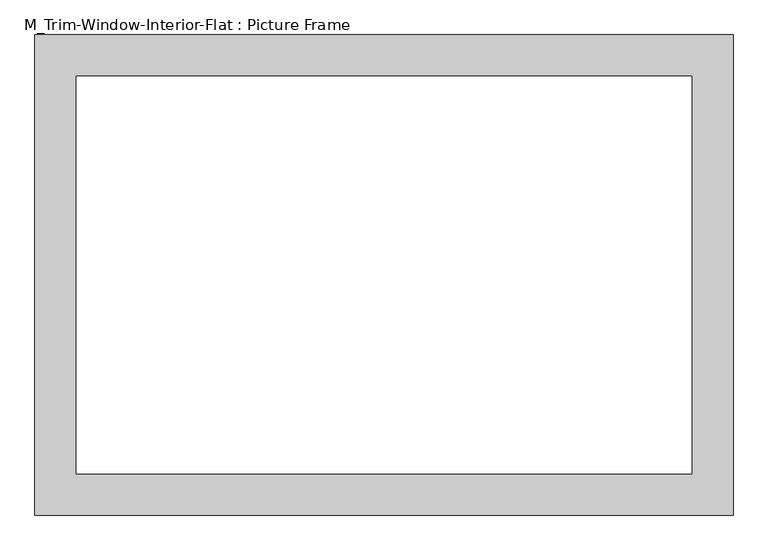
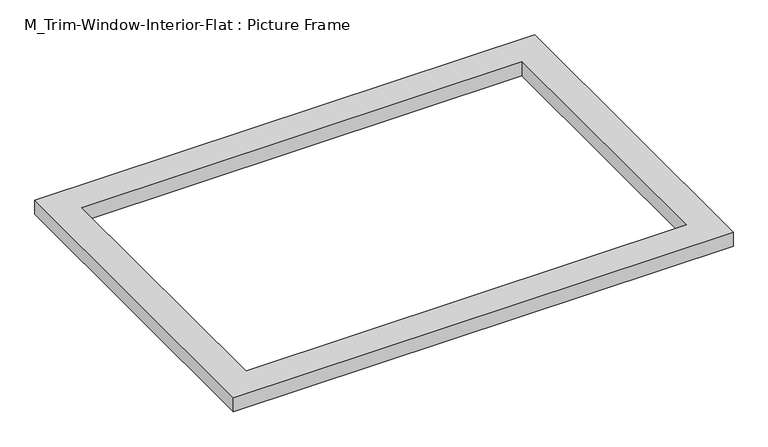
"""IFC4 building model written with IfcOpenShell, lengths in millimetres: proxy geometry, M_Trim-Window-Interior-Flat : Picture Frame."""

from ifc_helpers import new_model, si_unit, origin, origin_with_axes, place, context, project, spatial, polyline, outline, extrude, source, transform, mapped, element, save


def m_trim_window_interior_flat_picture_frame_87bc748b(model_context):
    return source(origin(), model_context, "Body", "SweptSolid", [
        extrude(outline(polyline([(504.5, 47.3), (504.5, -647.3), (-504.5, -647.3), (-504.5, 47.3), (504.5, 47.3)]), holes=[polyline([(444.5, -12.7), (-444.5, -12.7), (-444.5, -587.3), (444.5, -587.3), (444.5, -12.7)])]), origin_with_axes(), (0.0, 0.0, 1.0), 30.0),
    ])


if __name__ == "__main__":
    model = new_model("IFC4")
    model_context = context("Model", 3, world=origin())
    ifc_project = project(units=[si_unit("LENGTHUNIT", "METRE", prefix="MILLI")], contexts=[model_context])
    site = spatial("IfcSite", under=ifc_project)
    building = spatial("IfcBuilding", under=site)
    placement = place(None, origin())
    m_trim_window_interior_flat_picture_frame_shape = m_trim_window_interior_flat_picture_frame_87bc748b(model_context)
    element("IfcBuildingElementProxy", 1, Name="M_Trim-Window-Interior-Flat : Picture Frame", ObjectType="M_Trim-Window-Interior-Flat : Picture Frame", at=placement, inside=building, context=model_context, shape_type="MappedRepresentation", body=[
        mapped(m_trim_window_interior_flat_picture_frame_shape, transform((0.0, 0.0, 0.0), x_axis=(1.0, 0.0, 0.0), y_axis=(0.0, 1.0, 0.0), z_axis=(0.0, 0.0, 1.0))),
    ])
    save(model, "model.ifc")

# Revit data of these elements
# Type "M_Trim-Window-Interior-Flat : Picture Frame"
#   Trim Thickness_Picture Frame = 0' - 1.1811"
#   Trim Width = 0' - 2.3622"
#   Trim Thickness_with Sill = 0' - 0.7874"
#   Sill Thickness = 0' - 1.1811"
#   Opening Width [instance default] = 1' - 11.62205"
#   Opening Height [instance default] = 2' - 11.43307"
#   Default Elevation = 3' - 11.24409"
#   Sill = no
#   Picture Frame = yes
#   Trim Material [instance default] = none
# Element 1 (IfcBuildingElementProxy, "M_Trim-Window-Interior-Flat : Picture Frame")
#   Opening Width = 3' - 0"
#   Opening Height = 1' - 11.62205"
#   Trim Material = Wood - Stained
#   Materials on its faces: "Wood - Stained"
# Materials
#   "Wood - Stained": class "Wood", colour RGB 224 178 126, transparency 0, Cost = 0
